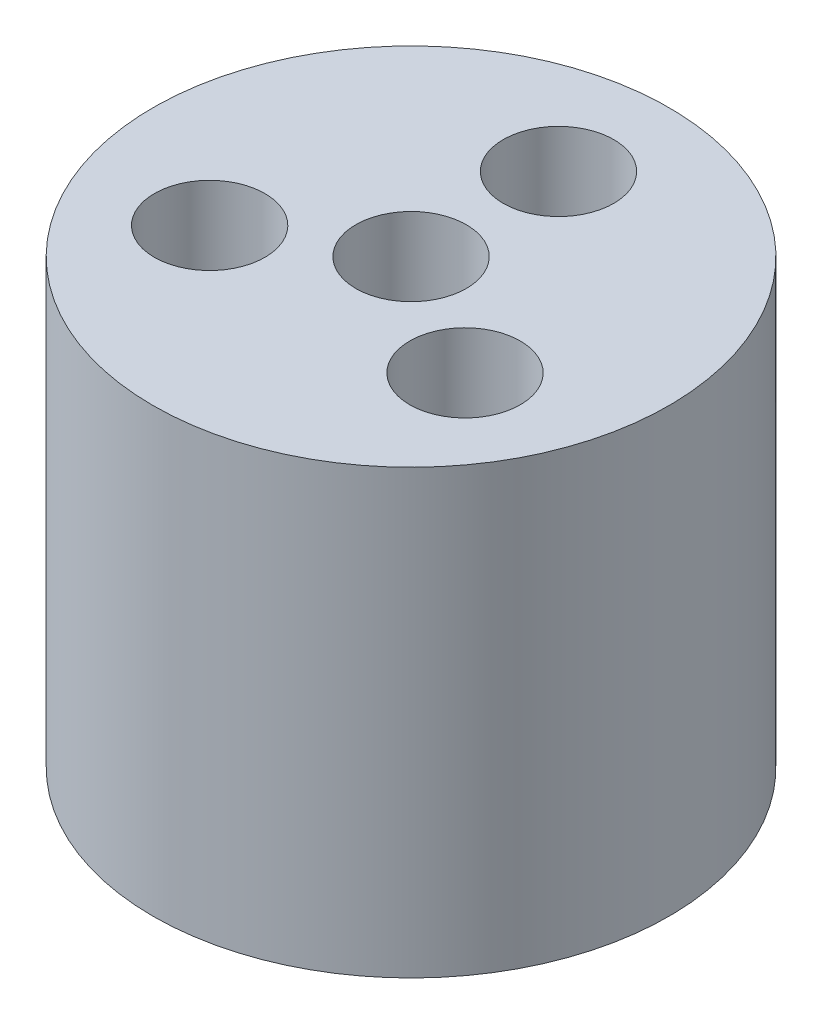
from build123d import *

# Parameters (mm, degrees)
CYLINDER_PROFILE_28_R           = 14
CYLINDER_BODY_28X24_DEPTH       = 24
HOLE_CIRCLE_SKETCH_3X_6_PCD16_R = 3
THROUGH_HOLES_3X_6_PCD16_DEPTH  = 29
CENTRE_HOLE_SKETCH_6_R          = 3
CENTRE_HOLE_6_DEPTH             = 29


with BuildPart() as part:
    # Cylinder Profile Ø28 → Cylinder Body Ø28x24 (new body)
    with BuildSketch(Plane(origin=(0, 0, 0), x_dir=(1, 0, 0), z_dir=(0, 1, 0))):
        with Locations(Location((0, 0, 0), (0, 0, 270))):
            Circle(CYLINDER_PROFILE_28_R)
    extrude(amount=CYLINDER_BODY_28X24_DEPTH)

    # Hole Circle Sketch 3xØ6 PCD16 → Through Holes 3xØ6 PCD16 (cut)
    with BuildSketch(Plane(origin=(0, 24, 0), x_dir=(1, 0, 0), z_dir=(0, 1, 0))):
        with Locations(Location((0, 8, 0), (0, 0, 270))):
            Circle(HOLE_CIRCLE_SKETCH_3X_6_PCD16_R)
        with Locations(Location((6.92820323, -4, 0), (0, 0, 270))):
            Circle(HOLE_CIRCLE_SKETCH_3X_6_PCD16_R)
        with Locations(Location((-6.92820323, -4, 0), (0, 0, 270))):
            Circle(HOLE_CIRCLE_SKETCH_3X_6_PCD16_R)
    extrude(amount=-THROUGH_HOLES_3X_6_PCD16_DEPTH, mode=Mode.SUBTRACT)

    # Centre Hole Sketch Ø6 → Centre Hole Ø6 (cut)
    with BuildSketch(Plane(origin=(0, 24, 0), x_dir=(1, 0, 0), z_dir=(0, 1, 0))):
        with Locations(Location((0, 0, 0), (0, 0, 270))):
            Circle(CENTRE_HOLE_SKETCH_6_R)
    extrude(amount=-CENTRE_HOLE_6_DEPTH, mode=Mode.SUBTRACT)


solid = part.part
